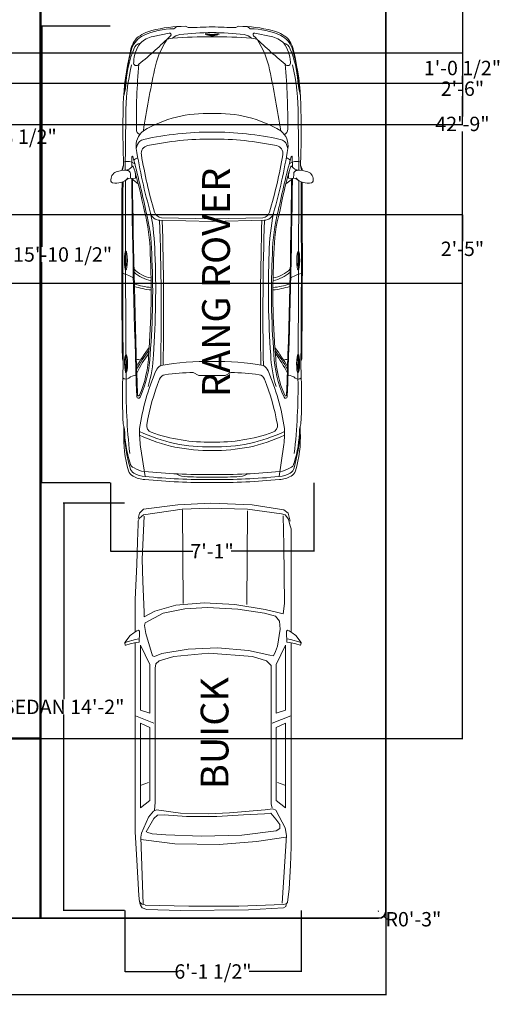
# Model space of a CAD drawing. Units: inches. Extents: x -56 to 545, y -536 to 185.
# Tile 4 of 7: x 345 to 545, y -531 to -120. Entities that reach past the tile are written whole.
import ezdxf

# ---------------------------------------------------------------- set-up
doc = ezdxf.new("R2010")
doc.units = ezdxf.units.IN
doc.header["$MEASUREMENT"] = 0
for name, color, linetype, lineweight in [('A-ANNO-DIMS', 2, 'Continuous', 18), ('A-ANNO-TEXT', 2, 'Continuous', 18), ('A-WALL', 7, 'Continuous', 50), ('C-PRKG-VEHI', 8, 'Continuous', 13), ('C-PROP', 7, 'Continuous', 35)]:
    doc.layers.add(name, color=color, linetype=linetype, lineweight=lineweight)
doc.styles.get("Standard").update_dxf_attribs({"font": 'arial.ttf'})
doc.dimstyles.get("Standard").update_dxf_attribs({"dimtxt": 6, "dimasz": 0.18, "dimexe": 0.18, "dimexo": 0.0625, "dimgap": 0.09, "dimtad": 0, "dimtih": 1, "dimtoh": 1, "dimdec": 0, "dimzin": 0, "dimdsep": 46, "dimlunit": 3, "dimtxsty": 'Standard', "dimcen": 0.09, "dimclrd": 3, "dimclre": 3, "dimclrt": 3, "dimadec": 0, "dimazin": 0, "dimtfac": 1, "dimtdec": 0, "dimtofl": 0, "dimtmove": 0, "dimatfit": 3, "dimfxl": 1, "dimtolj": 1, "dimtzin": 0, "dimarcsym": 0})

# ---------------------------------------------------------------- blocks, each defined once
blk = doc.blocks.new('A$C132F2E1D')
for p, q in [((0.543, 1.8886), (0.7013, 1.9079)), ((0.9043, 1.8866), (1.4518, 1.8937)), ((1.3706, 1.9103), (1.3631, 1.8926)), ((1.3631, 1.8926), (1.3631, 1.85)), ((1.407, 1.909), (1.4297, 1.9162)), ((1.4297, 1.9162), (1.4528, 1.9186)), ((3.3784, 1.9133), (3.3526, 1.9135)), ((3.3527, 1.9215), (3.3784, 1.9133)), ((3.3784, 1.9133), (3.5448, 1.9172)), ((4.008, 1.9136), (4.0609, 1.8993)), ((4.0895, 1.9062), (4.0345, 1.9064)), ((1.4203, 1.827), (1.3158, 1.8252)), ((1.3631, 1.85), (1.3696, 1.8261)), ((1.3696, 1.8261), (1.3875, 1.7961)), ((1.4882, 1.8409), (1.5335, 1.8395)), ((1.5342, 1.8622), (1.532, 1.7927)), ((1.5873, 1.7618), (1.5368, 1.8274)), ((2.5334, 1.8104), (2.5334, 1.8104)), ((4.24, 1.7387), (4.5389, 1.6933)), ((0.1023, 1.6121), (0.0698, 1.4487)), ((1.9298, 1.5286), (1.9419, 1.0174)), ((1.9544, 1.5457), (1.9669, 1.018)), ((0.0033, 1.3741), (0.0255, 1.4026)), ((0.12, 1.4158), (0.13, 1.4708)), ((0.0136, 1.2588), (0, 1.2857)), ((3.5213, 1.1507), (3.4897, 1.2072)), ((3.5213, 1.018), (3.5213, 1.1507)), ((0.0896, 1.018), (0.0719, 1.088)), ((0.0719, 1.088), (0.0821, 1.018)), ((0.0896, 1.018), (0.0719, 0.9479)), ((0.0719, 0.9479), (0.0821, 1.018)), ((0.1006, 1.018), (0.0828, 1.088)), ((0.0828, 1.088), (0.0931, 1.018)), ((0.1006, 1.018), (0.0828, 0.9479)), ((0.0828, 0.9479), (0.0931, 1.018)), ((1.9298, 0.5073), (1.9419, 1.0186)), ((1.9544, 0.4903), (1.9669, 1.018)), ((3.5213, 1.018), (3.5213, 0.8853)), ((3.5213, 0.8853), (3.4897, 0.8287)), ((0.0136, 0.7772), (0, 0.7503)), ((0.0033, 0.6619), (0.0255, 0.6334)), ((0.12, 0.6201), (0.13, 0.5651)), ((0.1023, 0.4239), (0.0698, 0.5873)), ((4.24, 0.2973), (4.5389, 0.3426)), ((1.4203, 0.209), (1.3158, 0.2108)), ((1.3631, 0.186), (1.3696, 0.2099)), ((1.3696, 0.2099), (1.3875, 0.2398)), ((1.5342, 0.1738), (1.532, 0.2432)), ((1.5873, 0.2742), (1.5368, 0.2086)), ((2.5334, 0.2256), (2.5334, 0.2256)), ((0.543, 0.1473), (0.7013, 0.128)), ((0.9043, 0.1493), (1.4518, 0.1422)), ((1.3631, 0.1434), (1.3631, 0.186)), ((1.3706, 0.1257), (1.3631, 0.1434)), ((1.407, 0.127), (1.4297, 0.1198)), ((1.4297, 0.1198), (1.4528, 0.1174)), ((1.4882, 0.1951), (1.5335, 0.1965)), ((3.3784, 0.1227), (3.3526, 0.1225)), ((3.3527, 0.1145), (3.3784, 0.1227)), ((3.3784, 0.1227), (3.5448, 0.1188)), ((4.008, 0.1224), (4.0609, 0.1367)), ((4.0895, 0.1298), (4.0345, 0.1295))]:
    blk.add_line(p, q)
for points in [[(0.5545, 1.882), (0.6265, 1.8906), (0.7013, 1.9079)], [(0.5545, 0.154), (0.6265, 0.1454), (0.7013, 0.128)]]:
    blk.add_lwpolyline(points)
for centre, radius, start, end in [((1.5478, 1.9486), 0.0885, 81.04298, 156.83016), ((1.3899, 1.9873), 0.191, 319.07376, 9.749), ((1.5584, 2.0162), 0.02, 9.749, 81.04298), ((0.7158, 0.1754), 1.7219, 95.75871, 106.66999), ((0.8722, -0.7564), 2.6698, 91.88228, 103.11637), ((0.8873, -0.259), 2.1457, 89.54661, 103.41209), ((1.0501, -7.5126), 9.4283, 87.83061, 91.61395), ((1.4598, 1.8405), 0.0865, 94.11262, 127.67305), ((1.357, 1.8976), 0.0949, 305.49305, 357.64193), ((1.7253, 1.8951), 0.2735, 161.16843, 183.85292), ((1.1259, -373.2553), 375.1468, 89.629132, 89.934477), ((2.3981, -110.3129), 112.2304, 89.512732, 90.424576), ((2.3135, -85.6642), 87.5918, 89.32026, 90.486182), ((2.845, 2.0124), 0.3681, 194.95147, 214.73189), ((3.7262, -4.5417), 6.4614, 87.50012, 91.60876), ((3.5093, 1.8853), 0.0477, 322.74562, 41.97986), ((4.047, 0.7351), 1.1643, 72.17211, 89.31712), ((4.1487, 0.7567), 1.151, 73.23925, 92.94622), ((3.9598, 0.0566), 1.8542, 74.63039, 85.98685), ((0.2968, 1.612), 0.2258, 109.40449, 154.47293), ((0.3163, 1.539), 0.3088, 99.30607, 129.20262), ((0.3712, 1.4803), 0.3273, 91.86492, 127.65559), ((0.2504, 1.7277), 0.0801, 105.04002, 171.6116), ((0.6164, 0.8965), 0.9874, 93.59221, 113.06049), ((0.3687, 1.7801), 0.0285, 298.61649, 106.64681), ((1.3159, 1.8202), 0.005, 90.9623, 254.9067), ((3.6251, 10.2904), 8.7843, 254.74992, 258.42395), ((1.3711, 1.7701), 0.0406, 119.08859, 187.71379), ((1.415, 1.8163), 0.005, 125.49305, 246.15831), ((1.526, 2.0675), 0.2796, 246.15831, 270.21376), ((1.4869, 1.8754), 0.0345, 177.75339, 272.27983), ((2.9375, 7.1081), 5.5139, 254.46339, 258.79798), ((1.527, 1.7929), 0.005, 270.21376, 358.17221), ((1.5189, 1.9076), 0.0394, 285.5168, 324.74311), ((0.383, -94.8685), 96.7028, 88.014877, 89.318555), ((0.383, -94.8685), 96.6953, 88.024999, 89.312887), ((2.2304, 1.5809), 0.311, 9.49373, 46.03765), ((2.2118, 1.5633), 0.3589, 10.99766, 42.14068), ((1.9842, 1.583), 0.6504, 4.23296, 19.62219), ((1.8364, 1.5439), 0.8263, 6.04716, 18.12027), ((3.6377, 1.7731), 0.1229, 137.35065, 175.10864), ((3.6347, -4.1374), 6.0215, 83.60515, 90.76636), ((4.3939, 1.7824), 0.0618, 20.2199, 81.07696), ((4.4332, 1.7639), 0.0825, 30.5014, 77.40713), ((4.2402, 1.6718), 0.2494, 6.73694, 31.93348), ((4.4497, 1.7647), 0.0991, 29.59344, 71.79345), ((4.2725, 1.6729), 0.2672, 4.38261, 29.81512), ((4.2692, 1.6755), 0.3003, 3.95205, 27.38435), ((0.7337, 1.4073), 0.7082, 154.75665, 180.37751), ((0.4002, 1.5413), 0.3661, 139.6653, 166.82313), ((-3.1006, 4.5928), 4.4926, 315.34452, 320.82807), ((0.3282, 1.5721), 0.2294, 133.18069, 169.95622), ((0.9479, -4.5143), 6.2948, 89.18041, 95.15468), ((3.0639, -11.0707), 12.9377, 98.94001, 101.70633), ((2.1201, 1.0748), 1.2415, 149.23442, 182.62114), ((1.0412, 1.7282), 0.0518, 20.25644, 93.59604), ((1.2013, 1.598), 0.1854, 80.28636, 142.92407), ((4.2615, 1.0246), 3.195, 167.7045, 180.11803), ((1.2818, 1.6513), 0.08, 80.41936, 168.20842), ((0.4389, -3.3422), 5.1841, 73.81498, 81.19317), ((0.4389, -3.3422), 5.1441, 73.81498, 80.41936), ((2.3151, 3.3892), 1.7486, 255.12579, 269.16493), ((4.2291, 0.3611), 1.6261, 119.33405, 127.48815), ((3.9957, 0.7394), 1.168, 117.24964, 128.49508), ((4.1001, 0.5643), 1.3548, 116.50327, 126.3201), ((3.2695, 2.7758), 1.1198, 271.90334, 293.67172), ((3.2695, 2.7758), 1.1348, 271.90334, 294.46129), ((3.5501, 1.7951), 0.1937, 184.16269, 197.14768), ((4.4219, -0.6417), 2.4183, 98.71867, 113.11099), ((3.7151, 1.7594), 0.01, 293.67172, 88.025), ((3.7322, 1.7588), 0.0175, 294.46129, 88.01488), ((4.0772, 0.45), 1.2989, 82.79642, 90.96292), ((2.6323, 1.0566), 1.6082, 358.62448, 25.49807), ((2.6328, 1.0566), 1.6427, 358.62433, 24.89552), ((-2.0942, 1.0548), 6.6138, 359.68361, 5.60781), ((-2.0924, 1.0548), 6.662, 359.68358, 5.50038), ((-2.0924, 1.0548), 6.692, 359.68359, 5.5002), ((1.3941, 1.2785), 1.3941, 165.61673, 179.7063), ((0.615, 0.7306), 0.885, 101.47468, 123.23035), ((4.2599, 1.0246), 3.1233, 168.11852, 180.1181), ((2.3151, 3.3892), 1.7636, 255.12579, 269.16493), ((1.8484, 1.5199), 0.0818, 6.1177, 72.66243), ((2.3534, 4.0946), 2.5026, 259.18744, 268.48682), ((1.861, 1.5459), 0.0934, 359.82686, 75.78413), ((2.6538, 10.9506), 9.3649, 267.75715, 274.02026), ((2.6795, 9.2996), 7.6836, 267.08589, 274.69152), ((2.6795, 9.2996), 7.6686, 267.08589, 274.69152), ((3.2609, 2.8713), 1.2635, 272.24484, 286.98853), ((4.4219, -0.6417), 2.3533, 99.98189, 111.58148), ((4.0261, 1.6071), 0.07, 19.45244, 99.98189), ((2.4672, 1.0516), 1.7249, 358.88416, 19.60736), ((2.8877, 30.3882), 28.8577, 268.14656, 271.05631), ((2.8877, 30.3882), 28.8827, 268.14933, 271.04617), ((5.6577, 1.1038), 2.2792, 169.08169, 182.15619), ((3.5126, 1.4843), 0.106, 112.12502, 151.18035), ((5.6068, 1.1784), 2.1173, 171.48298, 179.21912), ((3.582, 1.4816), 0.07, 111.58148, 171.48298), ((0.0845, 1.4458), 0.015, 168.75011, 315.34452), ((0.2091, 1.3272), 0.1256, 135.16316, 173.03669), ((4.4703, 1.065), 4.3644, 175.38888, 180.61666), ((2.4077, 1.0327), 2.3439, 172.40644, 180.3604), ((4.3309, 1.2705), 0.2103, 358.93016, 30.75657), ((-18.6368, 1.714), 18.656, 357.86205, 358.60201), ((-1.9281, 1.0543), 6.4726, 359.67956, 1.87886), ((-18.6368, 0.322), 18.656, 1.39799, 2.13795), ((2.4077, 1.0032), 2.3439, 179.6396, 187.59356), ((4.4703, 0.971), 4.3644, 179.38334, 184.61112), ((2.1201, 0.9612), 1.2415, 177.37886, 210.76558), ((4.2615, 1.0114), 3.195, 179.88197, 192.2955), ((4.2599, 1.0114), 3.1233, 179.8819, 191.88148), ((5.6577, 0.9322), 2.2792, 177.84381, 190.91831), ((2.6323, 0.9794), 1.6082, 334.50193, 1.37552), ((2.4672, 0.9844), 1.7249, 340.39264, 1.11584), ((2.6328, 0.9794), 1.6427, 335.10448, 1.37567), ((-2.0942, 0.9812), 6.6138, 354.39219, 0.31639), ((-2.0924, 0.9812), 6.662, 354.49962, 0.31642), ((-1.9281, 0.9816), 6.4726, 358.12114, 0.32044), ((-2.0924, 0.9812), 6.692, 354.4998, 0.31641), ((5.6068, 0.8576), 2.1173, 180.78088, 188.51702), ((1.3941, 0.7575), 1.3941, 180.2937, 194.38327), ((4.3309, 0.7655), 0.2103, 329.24343, 1.06984), ((0.7337, 0.6287), 0.7082, 179.62249, 205.24335), ((0.0845, 0.5902), 0.015, 44.65548, 191.24989), ((0.2091, 0.7087), 0.1256, 186.96331, 224.83684), ((-3.1006, -2.5569), 4.4926, 39.17193, 44.65548), ((0.615, 1.3054), 0.885, 236.76965, 258.52532), ((1.8484, 0.516), 0.0818, 287.33757, 353.8823), ((2.8877, -28.3523), 28.8577, 88.94369, 91.85344), ((2.8877, -28.3523), 28.8827, 88.95383, 91.85067), ((3.5126, 0.5516), 0.106, 208.81965, 247.87498), ((3.582, 0.5544), 0.07, 188.51702, 248.41852), ((0.4002, 0.4946), 0.3661, 193.17687, 220.3347), ((0.3282, 0.4639), 0.2294, 190.04378, 226.81931), ((3.0639, 13.1067), 12.9377, 258.29367, 261.05999), ((0.4389, 5.3782), 5.1841, 278.80683, 286.18502), ((0.4389, 5.3782), 5.1441, 279.58064, 286.18502), ((2.3151, -1.3533), 1.7636, 90.83507, 104.87421), ((1.861, 0.49), 0.0934, 284.21587, 0.17314), ((2.3534, -2.0587), 2.5026, 91.51318, 100.81256), ((2.6538, -8.9146), 9.3649, 85.97974, 92.24285), ((2.6795, -7.2636), 7.6836, 85.30848, 92.91411), ((2.6795, -7.2636), 7.6686, 85.30848, 92.91411), ((2.2304, 0.455), 0.311, 313.96235, 350.50627), ((2.2118, 0.4726), 0.3589, 317.85932, 349.00234), ((1.9842, 0.4529), 0.6504, 340.37781, 355.76704), ((1.8364, 0.4921), 0.8263, 341.87973, 353.95284), ((3.2609, -0.8353), 1.2635, 73.01147, 87.75516), ((4.4219, 2.6776), 2.4183, 246.88901, 261.28133), ((4.4219, 2.6776), 2.3533, 248.41852, 260.01811), ((4.0261, 0.4289), 0.07, 260.01811, 340.54756), ((0.2968, 0.424), 0.2258, 205.52707, 250.59551), ((1.2013, 0.438), 0.1854, 217.07593, 279.71364), ((1.2818, 0.3847), 0.08, 191.79158, 279.58064), ((3.6251, -8.2544), 8.7843, 101.57605, 105.25008), ((2.9375, -5.0721), 5.5139, 101.20202, 105.53661), ((2.3151, -1.3533), 1.7486, 90.83507, 104.87421), ((4.2291, 1.6749), 1.6261, 232.51185, 240.66595), ((3.9957, 1.2965), 1.168, 231.50492, 242.75036), ((4.1001, 1.4717), 1.3548, 233.6799, 243.49673), ((3.2695, -0.7398), 1.1198, 66.32828, 88.09666), ((3.2695, -0.7398), 1.1348, 65.53871, 88.09666), ((3.5501, 0.2409), 0.1937, 162.85232, 175.83731), ((4.2402, 0.3642), 0.2494, 328.06652, 353.26306), ((4.2725, 0.363), 0.2672, 330.18488, 355.61739), ((4.2692, 0.3605), 0.3003, 332.61565, 356.04795), ((0.3163, 0.497), 0.3088, 230.79738, 260.69393), ((0.3712, 0.5557), 0.3273, 232.34441, 268.13508), ((0.2504, 0.3083), 0.0801, 188.3884, 254.95998), ((0.7158, 1.8606), 1.7219, 253.33001, 264.24129), ((0.6164, 1.1394), 0.9874, 246.93951, 266.40779), ((0.3687, 0.2559), 0.0285, 253.35319, 61.38351), ((0.9479, 6.5502), 6.2948, 264.84532, 270.81959), ((0.8873, 2.295), 2.1457, 256.58791, 270.45339), ((1.0412, 0.3078), 0.0518, 266.40396, 339.74356), ((1.3159, 0.2158), 0.005, 105.0933, 269.0377), ((1.3711, 0.2659), 0.0406, 172.28621, 240.91141), ((1.415, 0.2196), 0.005, 113.84169, 234.50695), ((1.357, 0.1383), 0.0949, 2.35807, 54.50695), ((1.526, -0.0316), 0.2796, 89.78624, 113.84169), ((1.527, 0.2431), 0.005, 1.82779, 89.78624), ((0.383, 96.9045), 96.7028, 270.681445, 271.985123), ((0.383, 96.9045), 96.6953, 270.687113, 271.975001), ((2.845, 0.0236), 0.3681, 145.26811, 165.04853), ((3.6377, 0.2629), 0.1229, 184.89136, 222.64935), ((3.7151, 0.2766), 0.01, 271.975, 66.32828), ((3.7322, 0.2772), 0.0175, 271.98512, 65.53871), ((4.0772, 1.5859), 1.2989, 269.03708, 277.20358), ((4.3939, 0.2536), 0.0618, 278.92304, 339.7801), ((4.4332, 0.2721), 0.0825, 282.59287, 329.4986), ((4.4497, 0.2713), 0.0991, 288.20655, 330.40656), ((0.8722, 2.7923), 2.6698, 256.88363, 268.11772), ((1.0501, 9.5485), 9.4283, 268.38605, 272.16939), ((1.4598, 0.1954), 0.0865, 232.32695, 265.88738), ((1.7253, 0.1409), 0.2735, 176.14708, 198.83157), ((1.4869, 0.1606), 0.0345, 87.72017, 182.24661), ((1.5189, 0.1283), 0.0394, 35.25689, 74.4832), ((1.3899, 0.0487), 0.191, 350.251, 40.92624), ((1.1259, 375.2913), 375.1468, 270.065523, 270.370868), ((2.3981, 112.3489), 112.2304, 269.575424, 270.487268), ((2.3135, 87.7001), 87.5918, 269.513818, 270.67974), ((3.5093, 0.1507), 0.0477, 318.02014, 37.25438), ((3.7262, 6.5777), 6.4614, 268.39124, 272.49988), ((3.6347, 6.1734), 6.0215, 269.23364, 276.39485), ((4.047, 1.3009), 1.1643, 270.68288, 287.82789), ((3.9598, 1.9794), 1.8542, 274.01315, 285.36961), ((4.1487, 1.2793), 1.151, 267.05378, 286.76075), ((1.5478, 0.0874), 0.0885, 203.16984, 278.95702), ((1.5584, 0.0197), 0.02, 278.95702, 350.251)]:
    blk.add_arc(centre, radius, start, end)
for centre, major_axis in [((2.3605, 1.8864), (0.0938, -0.0005)), ((2.3473, 1.8864), (0.0703, -0.0004)), ((3.401, 1.8845), (0.0938, -0.0005)), ((3.3878, 1.8845), (0.0703, -0.0004))]:
    blk.add_ellipse(centre, major_axis=major_axis, ratio=0.16097)
at = {"extrusion": (0, 0, -1)}
for centre, major_axis in [((2.3605, 0.1496), (0.0938, 0.0005)), ((2.3473, 0.1495), (0.0703, 0.0004)), ((3.401, 0.1515), (0.0938, 0.0005)), ((3.3878, 0.1514), (0.0703, 0.0004))]:
    blk.add_ellipse(centre, major_axis=major_axis, ratio=0.16097, dxfattribs=at)
for points in [[(1.1398, 1.7049), (1.1459, 1.7208), (1.1615, 1.7621), (1.2055, 1.7737), (1.2326, 1.7808)], [(1.1398, 0.331), (1.1459, 0.3151), (1.1615, 0.2739), (1.2055, 0.2623), (1.2326, 0.2552)]]:
    blk.add_open_spline(points, degree=3, knots=[0, 0, 0, 0, 0.0487, 0.1263518, 0.1263518, 0.1263518, 0.1263518])
blk = doc.blocks.new('A$C381B4D24')
for p, q in [((-0.212, 1.042), (-0.142, 1.096)), ((-0.133, 1.095), (-0.162, 0.981)), ((-0.142, 1.096), (-0.127, 1.108)), ((-0.12, 1.108), (-0.133, 1.095)), ((-0.127, 1.108), (-0.12, 1.108)), ((-0.119, 1.108), (-0.097, 1.101)), ((-0.097, 1.095), (-0.11, 1.042)), ((-0.097, 1.101), (-0.097, 1.095)), ((-1.719, 0.898), (-1.68, 0.953)), ((-1.68, 0.953), (-1.583, 0.977)), ((-1.658, 0.914), (-1.605, 0.955)), ((-1.605, 0.955), (-1.538, 0.971)), ((-1.538, 0.971), (-1.491, 0.987)), ((-1.491, 0.987), (-0.253, 0.987)), ((-0.274, 0.942), (-0.269, 0.963)), ((-0.269, 0.963), (-0.244, 1.001)), ((-0.244, 1.001), (-0.212, 1.042)), ((-0.162, 0.981), (-0.17, 0.938)), ((-0.128, 0.963), (-0.131, 0.936)), ((-0.124, 0.989), (-0.128, 0.963)), ((-0.11, 1.042), (-0.124, 0.989)), ((-0.124, 0.987), (2.324, 0.987)), ((0.753, 0.983), (0.838, 0.761)), ((2.324, 0.987), (2.546, 0.978)), ((2.546, 0.978), (2.826, 0.963)), ((2.826, 0.963), (2.989, 0.944)), ((-1.777, 0.52), (-1.719, 0.898)), ((-1.725, 0.465), (-1.672, 0.873)), ((-1.672, 0.873), (-1.658, 0.914)), ((-1.293, 0.898), (-1.648, 0.89)), ((-0.596, 0.906), (-1.293, 0.898)), ((-0.473, 0.89), (-0.596, 0.906)), ((-0.524, 0.677), (-0.486, 0.827)), ((-0.486, 0.827), (-0.473, 0.89)), ((-0.442, 0.801), (-0.383, 0.849)), ((-0.383, 0.849), (-0.286, 0.856)), ((-0.286, 0.856), (-0.085, 0.825)), ((-0.269, 0.935), (-0.274, 0.942)), ((-0.263, 0.932), (-0.269, 0.935)), ((-0.246, 0.932), (-0.263, 0.932)), ((-0.131, 0.936), (-0.246, 0.932)), ((0.682, 0.92), (-0.097, 0.92)), ((-0.097, 0.92), (0.136, 0.809)), ((0.721, 0.809), (0.682, 0.92)), ((0.838, 0.92), (1.857, 0.92)), ((0.89, 0.809), (0.838, 0.92)), ((1.585, 0.912), (1.552, 0.825)), ((1.857, 0.92), (1.766, 0.809)), ((1.885, 0.802), (1.961, 0.844)), ((1.961, 0.844), (2.095, 0.916)), ((1.99, 0.802), (2.054, 0.852)), ((2.054, 0.852), (2.101, 0.852)), ((2.095, 0.916), (2.188, 0.93)), ((2.101, 0.852), (2.13, 0.809)), ((2.188, 0.93), (2.998, 0.88)), ((2.206, 0.923), (2.258, 0.574)), ((2.989, 0.944), (3.007, 0.929)), ((2.998, 0.93), (3.039, 0.923)), ((3.007, 0.929), (3.015, 0.893)), ((3.015, 0.893), (3.033, 0.361)), ((3.039, 0.923), (3.056, 0.894)), ((3.056, 0.894), (3.08, 0.475)), ((-0.481, 0.666), (-0.442, 0.801)), ((-0.085, 0.825), (-0.019, 0.801)), ((0.026, 0.73), (-0.033, 0.476)), ((-0.019, 0.801), (0.032, 0.777)), ((0.032, 0.777), (0.026, 0.73)), ((0.091, 0.69), (0.149, 0.746)), ((0.136, 0.809), (0.721, 0.809)), ((0.149, 0.746), (1.812, 0.746)), ((1.766, 0.809), (0.89, 0.809)), ((1.812, 0.746), (1.857, 0.761)), ((1.868, 0.766), (1.885, 0.802)), ((1.879, 0.674), (1.868, 0.766)), ((1.92, 0.745), (1.99, 0.802)), ((1.926, 0.666), (1.92, 0.745)), ((2.13, 0.809), (2.182, 0.396)), ((-0.583, 0.314), (-0.524, 0.677)), ((-0.526, 0.349), (-0.481, 0.666)), ((0.039, 0.523), (0.091, 0.69)), ((1.914, 0.247), (1.879, 0.674)), ((1.938, 0.417), (1.926, 0.666)), ((-1.797, 0.023), (-1.777, 0.52)), ((-0.033, 0.476), (-0.065, 0.103)), ((0, 0), (0.039, 0.523)), ((2.258, 0.574), (2.293, 0.126)), ((3.08, 0.475), (3.085, -0.344)), ((-1.738, 0), (-1.725, 0.465)), ((-1.706, 0.464), (-0.583, 0.456)), ((1.961, 0.097), (1.938, 0.417)), ((2.182, 0.396), (2.194, -0.088)), ((3.033, 0.361), (3.033, -0.237)), ((-0.602, -0.056), (-0.583, 0.314)), ((-0.546, -0.016), (-0.526, 0.349)), ((1.926, -0.009), (1.914, 0.247)), ((2.293, 0.126), (2.287, -0.408)), ((-1.777, -0.371), (-1.797, 0.023)), ((-1.725, -0.318), (-1.738, 0)), ((-0.065, 0.103), (-0.046, -0.246)), ((0.039, -0.42), (0, 0)), ((1.961, -0.265), (1.961, 0.097)), ((-0.576, -0.395), (-0.602, -0.056)), ((-0.533, -0.286), (-0.546, -0.016)), ((1.92, -0.337), (1.926, -0.009)), ((2.194, -0.088), (2.177, -0.514)), ((-1.658, -0.783), (-1.725, -0.318)), ((-1.719, -0.316), (-0.596, -0.308)), ((-0.481, -0.547), (-0.533, -0.286)), ((-0.046, -0.246), (0.006, -0.563)), ((1.879, -0.628), (1.92, -0.337)), ((1.938, -0.536), (1.961, -0.265)), ((3.033, -0.237), (3.021, -0.764)), ((3.085, -0.344), (3.074, -0.742)), ((-1.726, -0.782), (-1.777, -0.371)), ((-0.505, -0.648), (-0.576, -0.395)), ((0.091, -0.595), (0.039, -0.42)), ((2.287, -0.408), (2.241, -0.749)), ((-0.364, -0.761), (-0.481, -0.547)), ((0.006, -0.563), (0.039, -0.65)), ((1.943, -0.614), (1.938, -0.536)), ((2.177, -0.514), (2.165, -0.678)), ((-0.434, -0.774), (-0.505, -0.648)), ((0.032, -0.674), (-0.234, -0.753)), ((-0.097, -0.817), (0.136, -0.706)), ((0.039, -0.65), (0.032, -0.674)), ((0.13, -0.634), (0.091, -0.595)), ((0.182, -0.642), (0.13, -0.634)), ((0.136, -0.706), (0.721, -0.706)), ((1.793, -0.642), (0.182, -0.642)), ((0.721, -0.706), (0.682, -0.817)), ((0.753, -0.88), (0.838, -0.658)), ((0.89, -0.706), (0.838, -0.817)), ((1.766, -0.706), (0.89, -0.706)), ((1.857, -0.817), (1.766, -0.706)), ((1.883, -0.65), (1.793, -0.642)), ((1.897, -0.664), (1.879, -0.628)), ((1.967, -0.721), (1.897, -0.664)), ((1.984, -0.657), (1.943, -0.614)), ((2.142, -0.749), (1.984, -0.657)), ((2.165, -0.678), (2.147, -0.742)), ((-1.68, -0.829), (-1.726, -0.782)), ((-1.618, -0.832), (-1.658, -0.783)), ((-1.642, -0.774), (-1.125, -0.797)), ((-1.125, -0.797), (-0.86, -0.789)), ((-0.86, -0.789), (-0.492, -0.774)), ((-0.492, -0.774), (-0.434, -0.774)), ((-0.331, -0.769), (-0.364, -0.761)), ((-0.234, -0.753), (-0.331, -0.769)), ((0.682, -0.817), (-0.097, -0.817)), ((0.838, -0.817), (1.857, -0.817)), ((1.585, -0.809), (1.552, -0.722)), ((2.095, -0.778), (1.967, -0.721)), ((2.159, -0.806), (2.095, -0.778)), ((2.206, -0.813), (2.159, -0.806)), ((3.01, -0.785), (2.206, -0.813)), ((2.241, -0.749), (2.235, -0.813)), ((3.01, -0.803), (2.981, -0.829)), ((3.021, -0.82), (2.998, -0.828)), ((3.017, -0.764), (3.01, -0.803)), ((3.056, -0.799), (3.021, -0.82)), ((3.074, -0.742), (3.056, -0.799)), ((-1.616, -0.845), (-1.68, -0.829)), ((-1.585, -0.848), (-1.618, -0.832)), ((-1.545, -0.848), (-1.585, -0.848)), ((-1.338, -0.856), (-1.545, -0.848)), ((-1.064, -0.864), (-1.338, -0.856)), ((-0.643, -0.881), (-1.064, -0.864)), ((-0.397, -0.881), (-0.643, -0.881)), ((-0.256, -0.881), (-0.397, -0.881)), ((-0.269, -0.834), (-0.274, -0.841)), ((-0.274, -0.841), (-0.269, -0.862)), ((-0.263, -0.831), (-0.269, -0.834)), ((-0.269, -0.862), (-0.244, -0.9)), ((-0.246, -0.831), (-0.263, -0.831)), ((-0.131, -0.835), (-0.246, -0.831)), ((-0.244, -0.9), (-0.212, -0.941)), ((-0.212, -0.941), (-0.142, -0.995)), ((-0.162, -0.88), (-0.17, -0.837)), ((-0.133, -0.994), (-0.162, -0.88)), ((-0.128, -0.862), (-0.131, -0.835)), ((-0.124, -0.889), (-0.128, -0.862)), ((1.703, -0.881), (-0.125, -0.881)), ((-0.11, -0.941), (-0.124, -0.889)), ((-0.097, -0.994), (-0.11, -0.941)), ((2.144, -0.881), (1.703, -0.881)), ((2.483, -0.864), (2.144, -0.881)), ((2.907, -0.837), (2.483, -0.864)), ((2.981, -0.829), (2.907, -0.837)), ((-0.142, -0.995), (-0.127, -1.007)), ((-0.12, -1.007), (-0.133, -0.994)), ((-0.127, -1.007), (-0.12, -1.007)), ((-0.119, -1.007), (-0.097, -1)), ((-0.097, -1), (-0.097, -0.994))]:
    blk.add_line(p, q)
blk = doc.blocks.new('*D43')
at = {"layer": 'A-ANNO-DIMS', "color": 3, "lineweight": -2, "transparency": 16777216}
for p, q in [((222.25, -159.22), (222.25, -168.83)), ((285.57, -159.22), (285.57, -168.83)), ((222.43, -168.65), (285.39, -168.65)), ((285.57, -168.65), (285.75, -168.65))]:
    blk.add_line(p, q, dxfattribs=at)
at = {"layer": 'A-ANNO-DIMS', "color": 3, "transparency": 16777216}
for points in [[(222.43, -168.62), (222.43, -168.68), (222.25, -168.65)], [(285.39, -168.62), (285.39, -168.68), (285.57, -168.65)]]:
    blk.add_solid(points, dxfattribs=at)
at = {"layer": 'Defpoints', "color": 0, "transparency": 16777216}
for p in [(222.25, -159.15), (285.57, -159.15), (285.57, -168.65)]:
    blk.add_point(p, dxfattribs=at)
at = {"layer": 'A-ANNO-DIMS', "color": 3, "transparency": 16777216, "insert": (323.96, -168.65), "char_height": 6, "attachment_point": 5}
blk.add_mtext('\\A1;LOVESEAT 5\'-3 1/2"', dxfattribs=at)
blk = doc.blocks.new('*D47')
at = {"layer": 'A-ANNO-DIMS', "color": 3, "lineweight": -2, "transparency": 16777216}
for p, q in [((383.09, -122.58), (354.39, -122.58)), ((354.57, -122.76), (354.57, -214.63)), ((354.57, -312.89), (354.57, -221.02)), ((383.09, -313.07), (354.39, -313.07))]:
    blk.add_line(p, q, dxfattribs=at)
at = {"layer": 'A-ANNO-DIMS', "color": 3, "transparency": 16777216}
for points in [[(354.54, -122.76), (354.6, -122.76), (354.57, -122.58)], [(354.54, -312.89), (354.6, -312.89), (354.57, -313.07)]]:
    blk.add_solid(points, dxfattribs=at)
at = {"layer": 'Defpoints', "color": 0, "transparency": 16777216}
for p in [(383.15, -122.58), (354.57, -313.07), (383.15, -313.07)]:
    blk.add_point(p, dxfattribs=at)
at = {"layer": 'A-ANNO-DIMS', "color": 3, "transparency": 16777216, "insert": (354.57, -217.82), "char_height": 6, "attachment_point": 5}
blk.add_mtext('\\A1;SUV 15\'-10 1/2"', dxfattribs=at)
blk = doc.blocks.new('*D48')
at = {"layer": 'A-ANNO-DIMS', "color": 3, "lineweight": -2, "transparency": 16777216}
for p, q in [((383.15, -313.13), (383.15, -341.82)), ((467.97, -313.13), (467.97, -341.82)), ((383.33, -341.64), (417.52, -341.64)), ((467.79, -341.64), (433.6, -341.64))]:
    blk.add_line(p, q, dxfattribs=at)
at = {"layer": 'A-ANNO-DIMS', "color": 3, "transparency": 16777216}
for points in [[(383.33, -341.61), (383.33, -341.67), (383.15, -341.64)], [(467.79, -341.61), (467.79, -341.67), (467.97, -341.64)]]:
    blk.add_solid(points, dxfattribs=at)
at = {"layer": 'Defpoints', "color": 0, "transparency": 16777216}
for p in [(383.15, -313.07), (467.97, -313.07), (467.97, -341.64)]:
    blk.add_point(p, dxfattribs=at)
at = {"layer": 'A-ANNO-DIMS', "color": 3, "transparency": 16777216, "insert": (425.56, -341.64), "char_height": 6, "attachment_point": 5}
blk.add_mtext('\\A1;7\'-1"', dxfattribs=at)
blk = doc.blocks.new('*D49')
at = {"layer": 'A-ANNO-DIMS', "color": 3, "lineweight": -2, "transparency": 16777216}
for p, q in [((389.1, -321.67), (363.5, -321.67)), ((363.68, -321.85), (363.68, -403.43)), ((363.68, -491.39), (363.68, -409.81)), ((389.1, -491.57), (363.5, -491.57))]:
    blk.add_line(p, q, dxfattribs=at)
at = {"layer": 'A-ANNO-DIMS', "color": 3, "transparency": 16777216}
for points in [[(363.65, -321.85), (363.71, -321.85), (363.68, -321.67)], [(363.65, -491.39), (363.71, -491.39), (363.68, -491.57)]]:
    blk.add_solid(points, dxfattribs=at)
at = {"layer": 'Defpoints', "color": 0, "transparency": 16777216}
for p in [(389.16, -321.67), (363.68, -491.57), (389.16, -491.57)]:
    blk.add_point(p, dxfattribs=at)
at = {"layer": 'A-ANNO-DIMS', "color": 3, "transparency": 16777216, "insert": (363.68, -406.62), "char_height": 6, "attachment_point": 5}
blk.add_mtext('\\A1;SEDAN 14\'-2"', dxfattribs=at)
blk = doc.blocks.new('*D50')
at = {"layer": 'A-ANNO-DIMS', "color": 3, "lineweight": -2, "transparency": 16777216}
for p, q in [((389.16, -491.63), (389.16, -517.23)), ((462.73, -491.63), (462.73, -517.23)), ((389.34, -517.05), (410.87, -517.05)), ((462.55, -517.05), (441.02, -517.05))]:
    blk.add_line(p, q, dxfattribs=at)
at = {"layer": 'A-ANNO-DIMS', "color": 3, "transparency": 16777216}
for points in [[(389.34, -517.02), (389.34, -517.08), (389.16, -517.05)], [(462.55, -517.02), (462.55, -517.08), (462.73, -517.05)]]:
    blk.add_solid(points, dxfattribs=at)
at = {"layer": 'Defpoints', "color": 0, "transparency": 16777216}
for p in [(389.16, -491.57), (462.73, -491.57), (462.73, -517.05)]:
    blk.add_point(p, dxfattribs=at)
at = {"layer": 'A-ANNO-DIMS', "color": 3, "transparency": 16777216, "insert": (425.95, -517.05), "char_height": 6, "attachment_point": 5}
blk.add_mtext('\\A1;6\'-1 1/2"', dxfattribs=at)
blk = doc.blocks.new('*D51')
at = {"layer": 'A-ANNO-DIMS', "color": 3, "lineweight": -2, "transparency": 16777216}
for p, q in [((498.03, -491.9), (498.03, -526.99)), ((-5.97, -494.9), (-5.97, -526.99)), ((-5.79, -526.81), (235.52, -526.81)), ((497.85, -526.81), (256.55, -526.81))]:
    blk.add_line(p, q, dxfattribs=at)
at = {"layer": 'A-ANNO-DIMS', "color": 3, "transparency": 16777216}
for points in [[(-5.79, -526.78), (-5.79, -526.84), (-5.97, -526.81)], [(497.85, -526.78), (497.85, -526.84), (498.03, -526.81)]]:
    blk.add_solid(points, dxfattribs=at)
at = {"layer": 'Defpoints', "color": 0, "transparency": 16777216}
for p in [(498.03, -491.84), (-5.97, -494.84), (498.03, -526.81)]:
    blk.add_point(p, dxfattribs=at)
at = {"layer": 'A-ANNO-DIMS', "color": 3, "transparency": 16777216, "insert": (246.03, -526.81), "char_height": 6, "attachment_point": 5}
blk.add_mtext('\\A1;42\'-0"', dxfattribs=at)
blk = doc.blocks.new('*D59')
at = {"layer": 'A-ANNO-DIMS', "color": 3, "lineweight": -2, "transparency": 16777216}
for p, q in [((142.13, -133.66), (530.18, -133.66)), ((530, -133.84), (530, -145.47)), ((530, -163.41), (530, -151.78)), ((122.1, -163.59), (530.18, -163.59))]:
    blk.add_line(p, q, dxfattribs=at)
at = {"layer": 'A-ANNO-DIMS', "color": 3, "transparency": 16777216}
for points in [[(529.97, -133.84), (530.03, -133.84), (530, -133.66)], [(529.97, -163.41), (530.03, -163.41), (530, -163.59)]]:
    blk.add_solid(points, dxfattribs=at)
at = {"layer": 'Defpoints', "color": 0, "transparency": 16777216}
for p in [(142.07, -133.66), (530, -133.66), (122.03, -163.59)]:
    blk.add_point(p, dxfattribs=at)
at = {"layer": 'A-ANNO-DIMS', "color": 3, "transparency": 16777216, "insert": (530, -148.63), "char_height": 6, "attachment_point": 5}
blk.add_mtext('\\A1;2\'-6"', dxfattribs=at)
blk = doc.blocks.new('*D77')
at = {"layer": 'A-ANNO-DIMS', "color": 3, "lineweight": -2, "transparency": 16777216}
for p, q in [((116.1, -201.08), (530.18, -201.08)), ((530, -201.26), (530, -212.31)), ((530, -229.66), (530, -218.61)), ((116.1, -229.84), (530.18, -229.84))]:
    blk.add_line(p, q, dxfattribs=at)
at = {"layer": 'A-ANNO-DIMS', "color": 3, "transparency": 16777216}
for points in [[(529.97, -201.26), (530.03, -201.26), (530, -201.08)], [(529.97, -229.66), (530.03, -229.66), (530, -229.84)]]:
    blk.add_solid(points, dxfattribs=at)
at = {"layer": 'Defpoints', "color": 0, "transparency": 16777216}
for p in [(116.03, -201.08), (530, -201.08), (116.03, -229.84)]:
    blk.add_point(p, dxfattribs=at)
at = {"layer": 'A-ANNO-DIMS', "color": 3, "transparency": 16777216, "insert": (530, -215.46), "char_height": 6, "attachment_point": 5}
blk.add_mtext('\\A1;2\'-5"', dxfattribs=at)
blk = doc.blocks.new('*D86')
at = {"layer": 'A-ANNO-DIMS', "color": 3, "lineweight": -2, "transparency": 16777216}
for p, q in [((33.56, -133.66), (530.18, -133.66)), ((530, -133.84), (530, -136.81)), ((530, -146.17), (530, -143.2)), ((27.48, -146.35), (530.18, -146.35))]:
    blk.add_line(p, q, dxfattribs=at)
at = {"layer": 'A-ANNO-DIMS', "color": 3, "transparency": 16777216}
for points in [[(529.97, -133.84), (530.03, -133.84), (530, -133.66)], [(529.97, -146.17), (530.03, -146.17), (530, -146.35)]]:
    blk.add_solid(points, dxfattribs=at)
at = {"layer": 'Defpoints', "color": 0, "transparency": 16777216}
for p in [(33.5, -133.66), (27.42, -146.35), (530, -146.35)]:
    blk.add_point(p, dxfattribs=at)
at = {"layer": 'A-ANNO-DIMS', "color": 3, "transparency": 16777216, "insert": (530, -140.01), "char_height": 6, "attachment_point": 5}
blk.add_mtext('\\A1;1\'-0 1/2"', dxfattribs=at)
blk = doc.blocks.new('*D91')
at = {"layer": 'A-ANNO-DIMS', "color": 3, "lineweight": -2, "transparency": 16777216}
for p, q in [((498.1, 93.16), (530.18, 93.16)), ((530, 92.98), (530, -160.19)), ((530, -419.66), (530, -166.49)), ((354.1, -419.84), (530.18, -419.84))]:
    blk.add_line(p, q, dxfattribs=at)
at = {"layer": 'A-ANNO-DIMS', "color": 3, "transparency": 16777216}
for points in [[(529.97, 92.98), (530.03, 92.98), (530, 93.16)], [(529.97, -419.66), (530.03, -419.66), (530, -419.84)]]:
    blk.add_solid(points, dxfattribs=at)
at = {"layer": 'Defpoints', "color": 0, "transparency": 16777216}
for p in [(498.03, 93.16), (354.03, -419.84), (530, -419.84)]:
    blk.add_point(p, dxfattribs=at)
at = {"layer": 'A-ANNO-DIMS', "color": 3, "transparency": 16777216, "insert": (530, -163.34), "char_height": 6, "attachment_point": 5}
blk.add_mtext('\\A1;42\'-9"', dxfattribs=at)
blk = doc.blocks.new('*D92')
at = {"layer": 'A-ANNO-DIMS', "color": 3, "lineweight": -2, "transparency": 16777216}
for p, q in [((494.94, -491.84), (495.12, -491.84)), ((495.03, -491.93), (495.03, -491.75)), ((498.43, -495.24), (497.28, -494.09)), ((498.61, -495.24), (498.43, -495.24))]:
    blk.add_line(p, q, dxfattribs=at)
at = {"layer": 'A-ANNO-DIMS', "color": 3, "transparency": 16777216}
blk.add_solid([(497.3, -494.07), (497.26, -494.11), (497.15, -493.96)], dxfattribs=at)
at = {"layer": 'Defpoints', "color": 0, "transparency": 16777216}
for p in [(495.03, -491.84), (497.15, -493.96)]:
    blk.add_point(p, dxfattribs=at)
at = {"layer": 'A-ANNO-DIMS', "color": 3, "transparency": 16777216, "insert": (509.54, -495.24), "char_height": 6, "attachment_point": 5}
blk.add_mtext('\\A1;R0\'-3"', dxfattribs=at)

msp = doc.modelspace()

# ---------------------------------------------------------------- linework, layer by layer
at = {"layer": 'A-WALL'}
for p, q in [((354.03, 84.16), (354.03, -494.84)), ((236.14, -419.84), (354.03, -419.84))]:
    msp.add_line(p, q, dxfattribs=at)
at = {"layer": 'C-PROP'}
for p, q in [((498.03, 93.16), (498.03, -491.84)), ((122.03, -494.84), (495.03, -494.84))]:
    msp.add_line(p, q, dxfattribs=at)
msp.add_arc((495.03, -491.84), 3, 270, 0, dxfattribs=at)

# ---------------------------------------------------------------- block references
at = {"layer": 'C-PRKG-VEHI', "rotation": 270}
for name, p, xscale, yscale, zscale in [('A$C132F2E1D', (383.41, -122.58), 41.40424265251211, 41.40424265251211, 41.40424265251211), ('A$C381B4D24', (424.19, -384.19), 34.80043455380857, 34.80043455380857, 34.80043455380857)]:
    msp.add_blockref(name, p, dxfattribs=dict(at, xscale=xscale, yscale=yscale, zscale=zscale))

# ---------------------------------------------------------------- texts
at = {"layer": 'A-ANNO-TEXT', "char_height": 11.5844, "attachment_point": 1, "rotation": 90}
for s, insert in [('{\\fArial|b1|i0|c0|p34;RANG ROVER}', (421.42, -277.31)), ('{\\fArial|b1|i0|c0|p34;BUICK}', (420.81, -440.89))]:
    msp.add_mtext_dynamic_manual_height_columns(s, width=2189.6751, gutter_width=57.92, heights=[0], dxfattribs=dict(at, insert=insert))

# ---------------------------------------------------------------- dimensions: what is measured, and where the dimension line sits
at = {"layer": 'A-ANNO-DIMS'}
for base, p1, p2, picture, middle in [((530, -419.84), (498.03, 93.16), (354.03, -419.84), '*D91', (530, -163.34)), ((530, -146.35), (33.5, -133.66), (27.42, -146.35), '*D86', (530, -140.01)), ((530, -133.66), (122.03, -163.59), (142.07, -133.66), '*D59', (530, -148.63)), ((530, -201.08), (116.03, -229.84), (116.03, -201.08), '*D77', (530, -215.46))]:
    dim = msp.add_linear_dim(base=base, p1=p1, p2=p2, angle=90, dimstyle='Standard', override={"dimdec": 1, "dimlfac": 1, "dimrnd": 0, "dimzin": 1, "dimdsep": 46, "dimlunit": 4, "dimfrac": 2}, dxfattribs=at)
    dim.commit()
    dim.dimension.update_dxf_attribs({"geometry": picture, "text_midpoint": middle})
for base, p1, p2, text, picture, middle in [((354.57, -313.07), (383.15, -122.58), (383.15, -313.07), 'SUV <>', '*D47', (354.57, -217.82)), ((363.68, -491.57), (389.16, -321.67), (389.16, -491.57), 'SEDAN <>', '*D49', (363.68, -406.62))]:
    dim = msp.add_linear_dim(base=base, p1=p1, p2=p2, angle=270, text=text, dimstyle='Standard', override={"dimdec": 1, "dimlfac": 1, "dimrnd": 0, "dimzin": 1, "dimdsep": 46, "dimlunit": 4, "dimfrac": 2}, dxfattribs=at)
    dim.commit()
    dim.dimension.update_dxf_attribs({"geometry": picture, "text_midpoint": middle})
dim = msp.add_linear_dim(base=(285.57, -168.65), p1=(222.25, -159.15), p2=(285.57, -159.15), text='LOVESEAT <>', dimstyle='Standard', override={"dimdec": 1, "dimlfac": 1, "dimrnd": 0, "dimzin": 1, "dimdsep": 46, "dimlunit": 4, "dimfrac": 2}, dxfattribs=at)
dim.commit()
dim.dimension.update_dxf_attribs({"geometry": '*D43', "text_midpoint": (323.96, -168.65)})
for base, p1, p2, picture, middle in [((467.97, -341.64), (383.15, -313.07), (467.97, -313.07), '*D48', (425.56, -341.64)), ((498.03, -526.81), (-5.97, -494.84), (498.03, -491.84), '*D51', (246.03, -526.81)), ((462.73, -517.05), (389.16, -491.57), (462.73, -491.57), '*D50', (425.95, -517.05))]:
    dim = msp.add_linear_dim(base=base, p1=p1, p2=p2, dimstyle='Standard', override={"dimdec": 1, "dimlfac": 1, "dimrnd": 0, "dimzin": 1, "dimdsep": 46, "dimlunit": 4, "dimfrac": 2}, dxfattribs=at)
    dim.commit()
    dim.dimension.update_dxf_attribs({"geometry": picture, "text_midpoint": middle})
dim = msp.add_radius_dim(center=(495.03, -491.84), mpoint=(497.15, -493.96), dimstyle='Standard', override={"dimdec": 1, "dimlfac": 1, "dimrnd": 0, "dimzin": 1, "dimdsep": 46, "dimlunit": 4, "dimfrac": 2}, dxfattribs=at)
dim.commit()
dim.dimension.update_dxf_attribs({"geometry": '*D92', "text_midpoint": (509.54, -495.24), "dimtype": 164})

doc.saveas('drawing.dxf')
